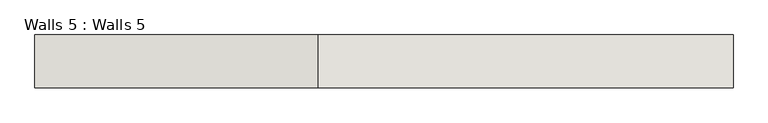
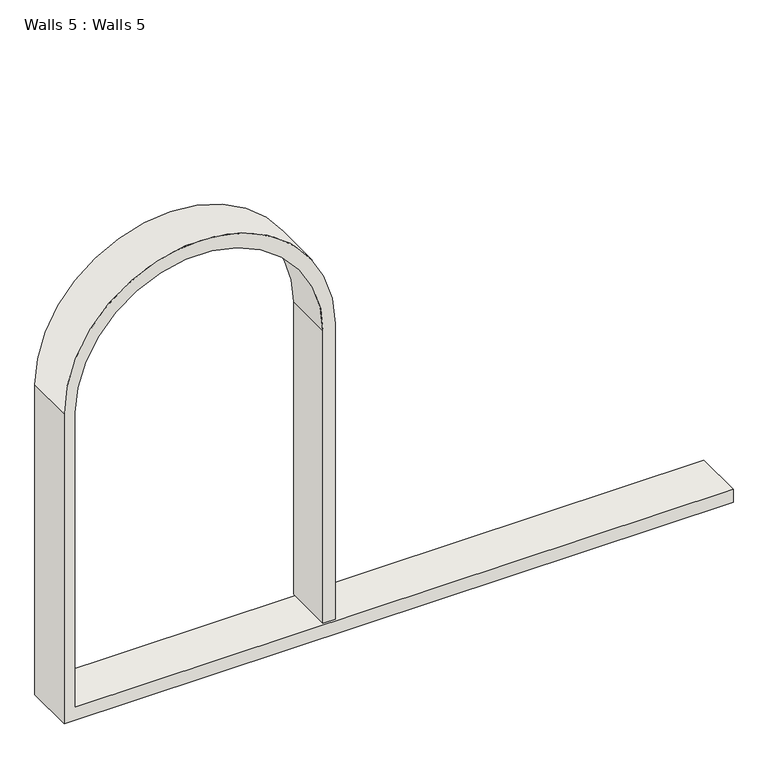
"""IFC4 building model written with IfcOpenShell, lengths in millimetres: wall geometry, Walls 5 : Walls 5."""

from ifc_helpers import new_model, si_unit, point, frame, frame_2d, origin, place, context, project, spatial, polyline, circle_curve, trimmed, segment, composite_curve, outline, extrude, source, transform, mapped, element, save


def walls_5_walls_5_0e1fe4ca(model_context):
    return source(origin(), model_context, "Body", "SweptSolid", [
        extrude(outline(composite_curve([segment(polyline([(6096.0, 3536.5665289), (6096.0, 7578.3159626), (6179.0195579, 7578.3159626), (6179.0195579, 3601.6943142), (8058.6195579, 3601.6943142)]), True, "CONTINUOUS"), segment(trimmed(circle_curve(frame_2d((8058.6195579, 4350.9943142)), 749.3), [point((8058.6195579, 3601.6943142))], [point((8058.6195579, 5100.2943142))], True, "CARTESIAN"), True, "CONTINUOUS"), segment(polyline([(8058.6195579, 5100.2943142), (6190.9217793, 5100.2943142), (6190.9217793, 5174.24434), (8077.2, 5174.24434)]), True, "CONTINUOUS"), segment(trimmed(circle_curve(frame_2d((8077.2, 4355.4054345)), 818.8389056), [point((8077.2, 5174.24434))], [point((8077.2, 3536.5665289))], False, "CARTESIAN"), True, "CONTINUOUS"), segment(polyline([(8077.2, 3536.5665289), (6096.0, 3536.5665289)]), True, "CONTINUOUS")], self_intersect=False)), frame((0.0, -1503.5851555, 0.0), z_axis=(0.0, 1.0, 0.0), x_axis=(0.0, 0.0, 1.0)), (0.0, 0.0, 1.0), 304.8),
    ])


if __name__ == "__main__":
    model = new_model("IFC4")
    model_context = context("Model", 3, world=origin())
    ifc_project = project(units=[si_unit("LENGTHUNIT", "METRE", prefix="MILLI")], contexts=[model_context])
    site = spatial("IfcSite", under=ifc_project)
    building = spatial("IfcBuilding", under=site)
    placement = place(None, origin())
    walls_5_walls_5_shape = walls_5_walls_5_0e1fe4ca(model_context)
    element("IfcWall", 1, ObjectType="Walls 5 : Walls 5", at=placement, inside=building, context=model_context, shape_type="MappedRepresentation", body=[
        mapped(walls_5_walls_5_shape, transform((0.0, 0.0, 0.0), x_axis=(1.0, 0.0, 0.0), y_axis=(0.0, 1.0, 0.0), z_axis=(0.0, 0.0, 1.0))),
    ])
    save(model, "model.ifc")

# Revit data of these elements
# Element 1 (IfcWall, "Walls 5 : Walls 5")
#   Materials on its faces: "Default Wall"
# Materials
#   "Default Wall": colour RGB 80 80 80, transparency 0
